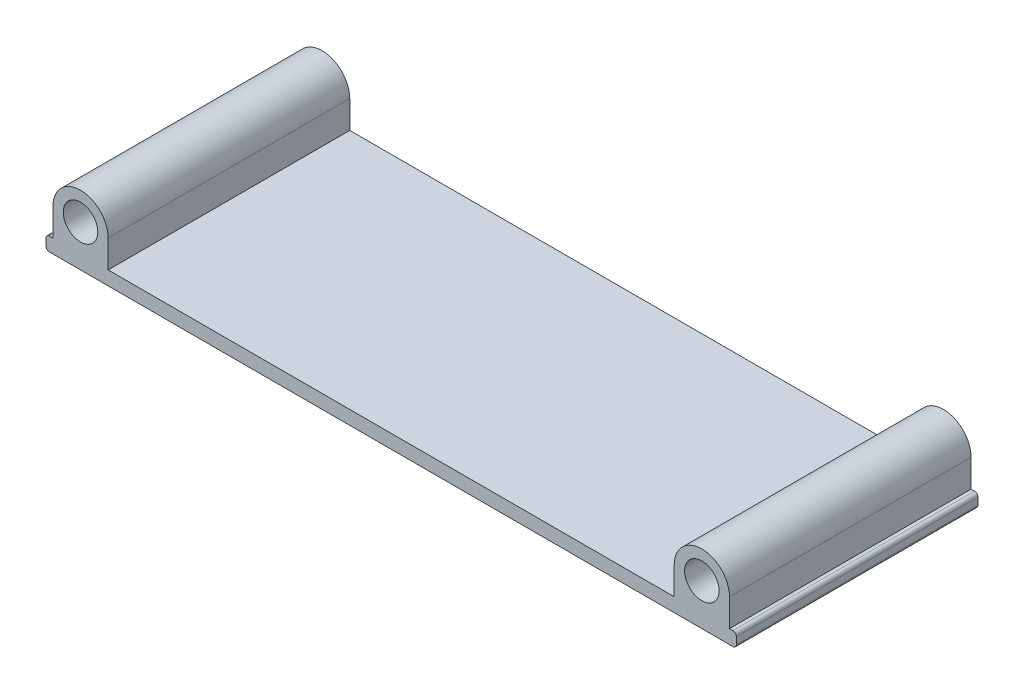
from build123d import *

# Parameters (mm, degrees)
ROLLED_EDGE_PLATE_PROFILE_R   = 2.5
ROLLED_EDGE_PLATE_PROFILE_W   = 82
ROLLED_EDGE_PLATE_PROFILE_H   = 2
ROLLED_EDGE_PLATE_PROFILE_W_2 = 1
ROLLED_EDGE_PLATE_PROFILE_W_3 = 8
PLATE_EXTRUDE_35MM_DEPTH      = 17.5
EDGE_FILLETS_R0_5_R           = 0.5


with BuildPart() as part:
    # Rolled Edge Plate Profile → Plate Extrude 35mm (new, symmetric)
    # profile 1 of 7: a face of its own
    with BuildSketch(Plane.XY):
        with BuildLine():
            Line((41, 5), (41, 1))
            Line((41, 1), (49, 1))
            Line((49, 1), (49, 5))
            ThreePointArc((49, 5), (45, 9), (41, 5))
        make_face()
        with Locations((45, 5)):
            Circle(ROLLED_EDGE_PLATE_PROFILE_R, mode=Mode.SUBTRACT)
    # profile 2 of 7: a face of its own
    with BuildSketch(Plane.XY):
        Rectangle(ROLLED_EDGE_PLATE_PROFILE_W, ROLLED_EDGE_PLATE_PROFILE_H)
    # profile 3 of 7: a face of its own
    with BuildSketch(Plane.XY):
        with Locations((49.5, 0)):
            Rectangle(ROLLED_EDGE_PLATE_PROFILE_W_2, ROLLED_EDGE_PLATE_PROFILE_H)
    # profile 4 of 7: a face of its own
    with BuildSketch(Plane.XY):
        with Locations((45, 0)):
            Rectangle(ROLLED_EDGE_PLATE_PROFILE_W_3, ROLLED_EDGE_PLATE_PROFILE_H)
    # profile 5 of 7: a face of its own
    with BuildSketch(Plane.XY):
        with Locations((-45, 0)):
            Rectangle(ROLLED_EDGE_PLATE_PROFILE_W_3, ROLLED_EDGE_PLATE_PROFILE_H)
    # profile 6 of 7: a face of its own
    with BuildSketch(Plane.XY):
        with Locations((-49.5, 0)):
            Rectangle(ROLLED_EDGE_PLATE_PROFILE_W_2, ROLLED_EDGE_PLATE_PROFILE_H)
    # profile 7 of 7: a face of its own
    with BuildSketch(Plane.XY):
        with BuildLine():
            Line((-49, 5), (-49, 1))
            Line((-49, 1), (-41, 1))
            Line((-41, 1), (-41, 5))
            ThreePointArc((-41, 5), (-45, 9), (-49, 5))
        make_face()
        with Locations((-45, 5)):
            Circle(ROLLED_EDGE_PLATE_PROFILE_R, mode=Mode.SUBTRACT)
    extrude(amount=PLATE_EXTRUDE_35MM_DEPTH, both=True)

    # Edge Fillets R0.5
    edge_fillets_r0_5_edges = [part.edges().sort_by_distance(p)[0] for p in [
        (50, 1, 0),
        (50, -1, 0),
        (-50, -1, 0),
        (-50, 1, 0),
    ]]
    fillet(edge_fillets_r0_5_edges, radius=EDGE_FILLETS_R0_5_R)


solid = part.part
